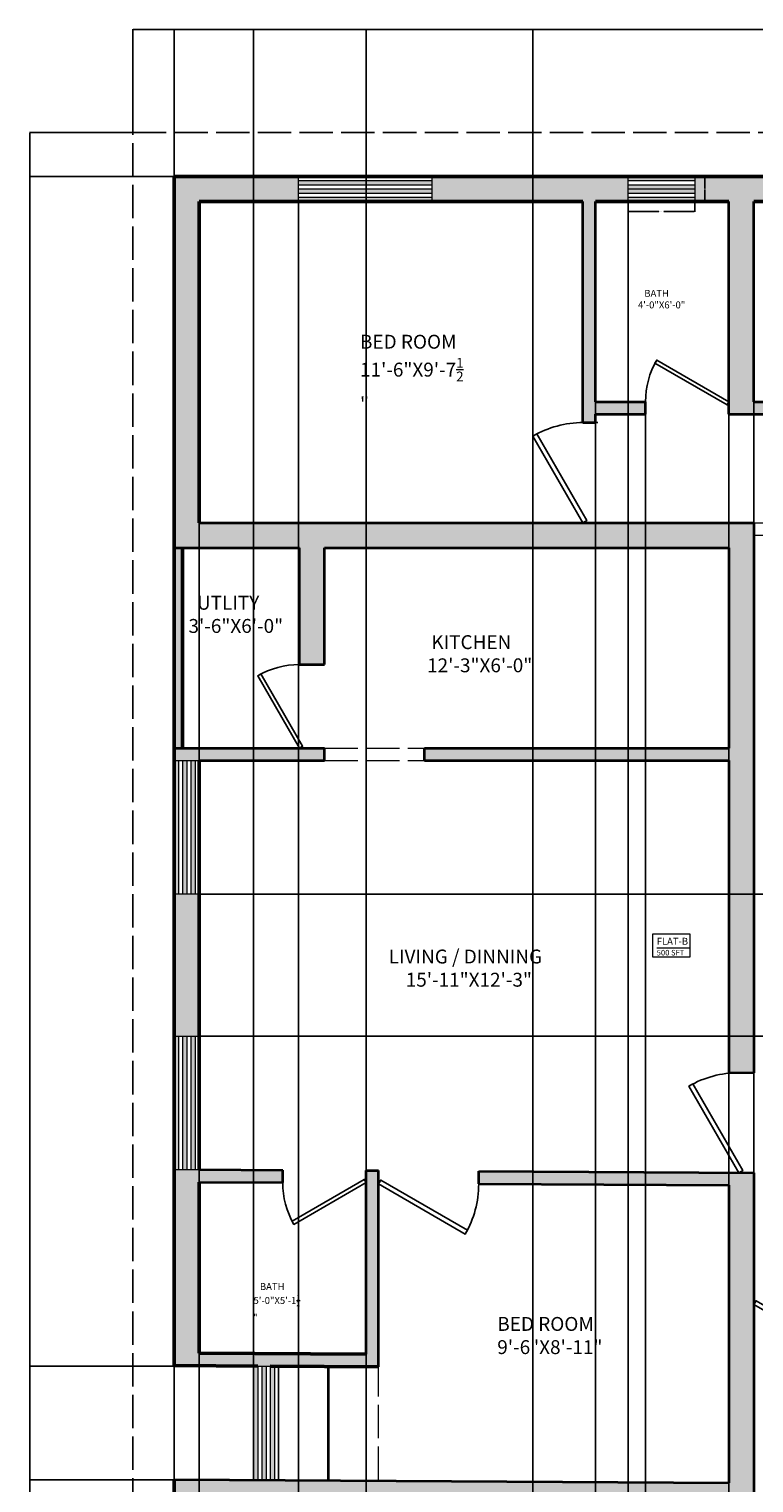
# Model space of a CAD drawing. Units: feet. Extents: x 2512 to 3087, y 1456 to 2266.
# Tile 3 of 5: x 2512 to 2773, y 1744 to 2266. Entities that reach past the tile are written whole.
import ezdxf

# ---------------------------------------------------------------- set-up
doc = ezdxf.new("R2010")
doc.units = ezdxf.units.FT
doc.linetypes.add('ACAD_ISO02W100', pattern=[15, 12, -3])
for name, color, linetype, lineweight in [('A-ANNO-DIMS', 2, 'Continuous', 18), ('A-AREA-IDEN', 7, 'Continuous', 18), ('A-DOOR', 240, 'Continuous', 25), ('A-GLAZ', 4, 'Continuous', 18), ('A-GLAZ-PATT', 252, 'Continuous', 13), ('A-WALL-OVHD', 8, 'ACAD_ISO02W100', 18), ('A-WALL-PATT', 252, 'Continuous', 13), ('ANNOTATION', 80, 'Continuous', 18), ('C-PROP', 8, 'ACAD_ISO02W100', 25), ('INNER WALL', 7, 'Continuous', 35), ('OPEN DOOR', 50, 'ACAD_ISO02W100', 18), ('OUTER WALL', 7, 'Continuous', 50)]:
    doc.layers.add(name, color=color, linetype=linetype, lineweight=lineweight)
doc.styles.get("Standard").update_dxf_attribs({"font": 'arial.ttf'})
doc.dimstyles.get("Standard").update_dxf_attribs({"dimtxt": 0.18, "dimasz": 0.18, "dimexe": 0.18, "dimexo": 0.0625, "dimgap": 0.09, "dimtad": 0, "dimtih": 1, "dimtoh": 1, "dimdec": 4, "dimzin": 0, "dimdsep": 46, "dimtxsty": 'Standard', "dimcen": 0.09, "dimadec": 0, "dimazin": 0, "dimtfac": 1, "dimtdec": 4, "dimtofl": 0, "dimtmove": 0, "dimatfit": 3, "dimfxl": 1, "dimtolj": 1, "dimtzin": 0, "dimarcsym": 0})

# ---------------------------------------------------------------- blocks, each defined once
blk = doc.blocks.new('*U8')
for p, q in [((0, 0), (0, 6)), ((40, 0), (40, 6))]:
    blk.add_line(p, q)
blk.add_lwpolyline([(0, 0), (34.64, -20), (35.52, -18.48), (0.87, 1.52)], close=True)
blk.add_arc((0, 0), 40, 330, 0)
blk = doc.blocks.new('*U3')
for p, q in [((0, 0), (0, 5)), ((40, 0), (40, 5))]:
    blk.add_line(p, q)
blk.add_lwpolyline([(0, 0), (34.64, -20), (35.52, -18.48), (0.87, 1.52)], close=True)
blk.add_arc((0, 0), 40, 330, 0)
blk = doc.blocks.new('*U4')
for p, q in [((-40, 0), (-40, 6)), ((0, 0), (0, 6))]:
    blk.add_line(p, q)
blk.add_lwpolyline([(0, 0), (-34.64, -20), (-35.52, -18.48), (-0.87, 1.52)], close=True)
blk.add_arc((0, 0), 40, 180, 210)
blk = doc.blocks.new('*U5')
for p, q in [((0, 0), (0, -6)), ((-40, 0), (-40, -6))]:
    blk.add_line(p, q)
blk.add_lwpolyline([(0, 0), (-34.64, 20), (-35.52, 18.48), (-0.88, -1.52)], close=True)
blk.add_arc((0, 0), 40, 150, 180)
blk = doc.blocks.new('*U6')
for p, q in [((-40, 0), (-40, 6)), ((0, 0), (0, 6))]:
    blk.add_line(p, q)
blk.add_lwpolyline([(0, 0), (-34.64, -20), (-35.52, -18.48), (-0.88, 1.52)], close=True)
blk.add_arc((0, 0), 40, 180, 210)
blk = doc.blocks.new('WIN-48IN')
h = blk.add_hatch(color=256)
h.dxf.hatch_style = 1
h.paths.add_polyline_path([(0, 7.5), (0, 6), (48, 6), (48, 7.5)])
h.paths.add_polyline_path([(48, 3), (48, 4.5), (0, 4.5), (0, 3)])
h.paths.add_polyline_path([(48, 0), (48, 1.5), (0, 1.5), (0, 0)])
for p, q in [((0, 9), (48, 9)), ((0, 0), (0, 9)), ((0, 7.5), (48, 7.5)), ((0, 6), (48, 6)), ((48, 9), (48, 0)), ((0, 4.5), (48, 4.5)), ((0, 4.5), (48, 4.5)), ((0, 3), (48, 3)), ((0, 1.5), (48, 1.5)), ((48, 0), (0, 0))]:
    blk.add_line(p, q)
blk = doc.blocks.new('VENT-24IN')
h = blk.add_hatch(color=256)
h.dxf.hatch_style = 1
h.paths.add_polyline_path([(24, 7.5), (24, 9), (0, 9), (0, 7.5)])
h.paths.add_polyline_path([(0, 1.5), (0, 0), (24, 0), (24, 1.5)])
h.paths.add_polyline_path([(0, 4.5), (0, 3), (24, 3), (24, 4.5)])
h.paths.add_polyline_path([(24, 4.5), (24, 6), (0, 6), (0, 4.5)])
for p, q in [((0, 9), (24, 9)), ((0, 0), (0, 9)), ((0, 7.5), (24, 7.5)), ((0, 6), (24, 6)), ((24, 9), (24, 0)), ((0, 4.5), (24, 4.5)), ((0, 3), (24, 3)), ((0, 1.5), (24, 1.5)), ((24, 0), (0, 0))]:
    blk.add_line(p, q)
blk = doc.blocks.new('FLAT-ID-FRAME')
blk.add_line((1.44, 3.36), (13.18, 3.36))
blk.add_lwpolyline([(0, 8.39), (13.37, 8.39), (13.37, 0), (0, 0)], close=True)
blk = doc.blocks.new('*D15')
at = {"layer": 'A-ANNO-DIMS', "color": 0, "lineweight": -2, "transparency": 16777216}
for p, q in [((2727.45, 2204.17), (2727.45, 2200.45)), ((2727.63, 2200.63), (2738.54, 2200.63)), ((2751.27, 2200.63), (2740.35, 2200.63)), ((2751.45, 2204.17), (2751.45, 2200.45))]:
    blk.add_line(p, q, dxfattribs=at)
at = {"layer": 'A-ANNO-DIMS', "color": 0, "transparency": 16777216}
for points in [[(2727.63, 2200.66), (2727.63, 2200.6), (2727.45, 2200.63)], [(2751.27, 2200.66), (2751.27, 2200.6), (2751.45, 2200.63)]]:
    blk.add_solid(points, dxfattribs=at)
at = {"layer": 'Defpoints', "color": 0, "transparency": 16777216}
for p in [(2727.45, 2204.23), (2751.45, 2204.23), (2751.45, 2200.63)]:
    blk.add_point(p, dxfattribs=at)
at = {"layer": 'A-ANNO-DIMS', "color": 0, "transparency": 16777216, "insert": (2739.45, 2200.63), "char_height": 0.18, "attachment_point": 5}
blk.add_mtext('\\A1;VENT 24 TYP.', dxfattribs=at)
blk = doc.blocks.new('*D16')
at = {"layer": 'A-ANNO-DIMS', "color": 0, "lineweight": -2, "transparency": 16777216}
for p, q in [((2751.51, 2213.23), (2755.23, 2213.23)), ((2755.05, 2213.05), (2755.05, 2208.91)), ((2755.05, 2204.41), (2755.05, 2208.55)), ((2751.51, 2204.23), (2755.23, 2204.23))]:
    blk.add_line(p, q, dxfattribs=at)
at = {"layer": 'A-ANNO-DIMS', "color": 0, "transparency": 16777216}
for points in [[(2755.02, 2213.05), (2755.08, 2213.05), (2755.05, 2213.23)], [(2755.02, 2204.41), (2755.08, 2204.41), (2755.05, 2204.23)]]:
    blk.add_solid(points, dxfattribs=at)
at = {"layer": 'Defpoints', "color": 0, "transparency": 16777216}
for p in [(2751.45, 2213.23), (2755.05, 2213.23), (2751.45, 2204.23)]:
    blk.add_point(p, dxfattribs=at)
at = {"layer": 'A-ANNO-DIMS', "color": 0, "transparency": 16777216, "insert": (2755.05, 2208.73), "char_height": 0.18, "attachment_point": 5}
blk.add_mtext('\\A1;9 TYP.', dxfattribs=at)
blk = doc.blocks.new('*D17')
at = {"layer": 'A-ANNO-DIMS', "color": 0, "lineweight": -2, "transparency": 16777216}
for p, q in [((2549.29, 2229.08), (2549.29, 2266.2)), ((2549.47, 2266.02), (2799.17, 2266.02)), ((3049.67, 2266.02), (2799.96, 2266.02)), ((3049.85, 2229.08), (3049.85, 2266.2))]:
    blk.add_line(p, q, dxfattribs=at)
at = {"layer": 'A-ANNO-DIMS', "color": 0, "transparency": 16777216}
for points in [[(2549.47, 2266.05), (2549.47, 2265.99), (2549.29, 2266.02)], [(3049.67, 2266.05), (3049.67, 2265.99), (3049.85, 2266.02)]]:
    blk.add_solid(points, dxfattribs=at)
at = {"layer": 'Defpoints', "color": 0, "transparency": 16777216}
for p in [(3049.85, 2266.02), (2549.29, 2229.02), (3049.85, 2229.02)]:
    blk.add_point(p, dxfattribs=at)
at = {"layer": 'A-ANNO-DIMS', "color": 0, "transparency": 16777216, "insert": (2799.57, 2266.02), "char_height": 0.18, "attachment_point": 5}
blk.add_mtext('\\A1;500.6', dxfattribs=at)
blk = doc.blocks.new('*D18')
at = {"layer": 'A-ANNO-DIMS', "color": 0, "lineweight": -2, "transparency": 16777216}
for p, q in [((2549.23, 2229.02), (2512.11, 2229.02)), ((2512.29, 2228.84), (2512.29, 1861.31)), ((2512.29, 1493.41), (2512.29, 1860.94)), ((2549.23, 1493.23), (2512.11, 1493.23))]:
    blk.add_line(p, q, dxfattribs=at)
at = {"layer": 'A-ANNO-DIMS', "color": 0, "transparency": 16777216}
for points in [[(2512.26, 2228.84), (2512.32, 2228.84), (2512.29, 2229.02)], [(2512.26, 1493.41), (2512.32, 1493.41), (2512.29, 1493.23)]]:
    blk.add_solid(points, dxfattribs=at)
at = {"layer": 'Defpoints', "color": 0, "transparency": 16777216}
for p in [(2512.29, 2229.02), (2549.29, 2229.02), (2549.29, 1493.23)]:
    blk.add_point(p, dxfattribs=at)
at = {"layer": 'A-ANNO-DIMS', "color": 0, "transparency": 16777216, "insert": (2512.29, 1861.13), "char_height": 0.18, "attachment_point": 5}
blk.add_mtext('\\A1;735.8', dxfattribs=at)
blk = doc.blocks.new('*D19')
at = {"layer": 'A-ANNO-DIMS', "color": 0, "lineweight": -2, "transparency": 16777216}
for p, q in [((2564.22, 2213.29), (2564.22, 2266.2)), ((2564.4, 2266.02), (2803.93, 2266.02)), ((3044.04, 2266.02), (2804.51, 2266.02)), ((3044.22, 2088.29), (3044.22, 2266.2))]:
    blk.add_line(p, q, dxfattribs=at)
at = {"layer": 'A-ANNO-DIMS', "color": 0, "transparency": 16777216}
for points in [[(2564.4, 2266.05), (2564.4, 2265.99), (2564.22, 2266.02)], [(3044.04, 2266.05), (3044.04, 2265.99), (3044.22, 2266.02)]]:
    blk.add_solid(points, dxfattribs=at)
at = {"layer": 'Defpoints', "color": 0, "transparency": 16777216}
for p in [(3044.22, 2266.02), (2564.22, 2213.23), (3044.22, 2088.23)]:
    blk.add_point(p, dxfattribs=at)
at = {"layer": 'A-ANNO-DIMS', "color": 0, "transparency": 16777216, "insert": (2804.22, 2266.02), "char_height": 0.18, "attachment_point": 5}
blk.add_mtext('\\A1;480', dxfattribs=at)
blk = doc.blocks.new('*D20')
at = {"layer": 'A-ANNO-DIMS', "color": 0, "lineweight": -2, "transparency": 16777216}
for p, q in [((2564.16, 2213.23), (2512.11, 2213.23)), ((2512.29, 2213.05), (2512.29, 1853.41)), ((2512.29, 1493.41), (2512.29, 1853.05)), ((2693.16, 1493.23), (2512.11, 1493.23))]:
    blk.add_line(p, q, dxfattribs=at)
at = {"layer": 'A-ANNO-DIMS', "color": 0, "transparency": 16777216}
for points in [[(2512.26, 2213.05), (2512.32, 2213.05), (2512.29, 2213.23)], [(2512.26, 1493.41), (2512.32, 1493.41), (2512.29, 1493.23)]]:
    blk.add_solid(points, dxfattribs=at)
at = {"layer": 'Defpoints', "color": 0, "transparency": 16777216}
for p in [(2512.29, 2213.23), (2564.22, 2213.23), (2693.22, 1493.23)]:
    blk.add_point(p, dxfattribs=at)
at = {"layer": 'A-ANNO-DIMS', "color": 0, "transparency": 16777216, "insert": (2512.29, 1853.23), "char_height": 0.18, "attachment_point": 5}
blk.add_mtext('\\A1;720', dxfattribs=at)
blk = doc.blocks.new('*D21')
at = {"layer": 'A-ANNO-DIMS', "color": 0, "lineweight": -2, "transparency": 16777216}
for p, q in [((2573.22, 2204.17), (2573.22, 1456.05)), ((2608.89, 2204.17), (2608.89, 1456.05)), ((2573.4, 1456.23), (2590.66, 1456.23)), ((2608.71, 1456.23), (2591.45, 1456.23))]:
    blk.add_line(p, q, dxfattribs=at)
at = {"layer": 'A-ANNO-DIMS', "color": 0, "transparency": 16777216}
for points in [[(2573.4, 1456.26), (2573.4, 1456.2), (2573.22, 1456.23)], [(2608.71, 1456.26), (2608.71, 1456.2), (2608.89, 1456.23)]]:
    blk.add_solid(points, dxfattribs=at)
at = {"layer": 'Defpoints', "color": 0, "transparency": 16777216}
for p in [(2573.22, 2204.23), (2608.89, 2204.23), (2608.89, 1456.23)]:
    blk.add_point(p, dxfattribs=at)
at = {"layer": 'A-ANNO-DIMS', "color": 0, "transparency": 16777216, "insert": (2591.05, 1456.23), "char_height": 0.18, "attachment_point": 5}
blk.add_mtext('\\A1;35.67', dxfattribs=at)
blk = doc.blocks.new('*D22')
at = {"layer": 'A-ANNO-DIMS', "color": 0, "lineweight": -2, "transparency": 16777216}
for p, q in [((2715.72, 2204.17), (2715.72, 1456.05)), ((2727.45, 2204.17), (2727.45, 1456.05)), ((2715.9, 1456.23), (2721.13, 1456.23)), ((2727.27, 1456.23), (2722.04, 1456.23))]:
    blk.add_line(p, q, dxfattribs=at)
at = {"layer": 'A-ANNO-DIMS', "color": 0, "transparency": 16777216}
for points in [[(2715.9, 1456.26), (2715.9, 1456.2), (2715.72, 1456.23)], [(2727.27, 1456.26), (2727.27, 1456.2), (2727.45, 1456.23)]]:
    blk.add_solid(points, dxfattribs=at)
at = {"layer": 'Defpoints', "color": 0, "transparency": 16777216}
for p in [(2715.72, 2204.23), (2727.45, 2204.23), (2727.45, 1456.23)]:
    blk.add_point(p, dxfattribs=at)
at = {"layer": 'A-ANNO-DIMS', "color": 0, "transparency": 16777216, "insert": (2721.58, 1456.23), "char_height": 0.18, "attachment_point": 5}
blk.add_mtext('\\A1;11.729', dxfattribs=at)
blk = doc.blocks.new('*D29')
at = {"layer": 'A-ANNO-DIMS', "color": 0, "lineweight": -2, "transparency": 16777216}
for p, q in [((2633.22, 1517.86), (2633.22, 2266.2)), ((2633.4, 2266.02), (2663, 2266.02)), ((2693.04, 2266.02), (2663.44, 2266.02)), ((2693.22, 1517.86), (2693.22, 2266.2))]:
    blk.add_line(p, q, dxfattribs=at)
at = {"layer": 'A-ANNO-DIMS', "color": 0, "transparency": 16777216}
for points in [[(2633.4, 2266.05), (2633.4, 2265.99), (2633.22, 2266.02)], [(2693.04, 2266.05), (2693.04, 2265.99), (2693.22, 2266.02)]]:
    blk.add_solid(points, dxfattribs=at)
at = {"layer": 'Defpoints', "color": 0, "transparency": 16777216}
for p in [(2693.22, 2266.02), (2633.22, 1517.8), (2693.22, 1517.8)]:
    blk.add_point(p, dxfattribs=at)
at = {"layer": 'A-ANNO-DIMS', "color": 0, "transparency": 16777216, "insert": (2663.22, 2266.02), "char_height": 0.18, "attachment_point": 5}
blk.add_mtext('\\A1;60', dxfattribs=at)
blk = doc.blocks.new('*D46')
at = {"layer": 'A-ANNO-DIMS', "color": 0, "lineweight": -2, "transparency": 16777216}
for p, q in [((2573.28, 1955.22), (3087.03, 1955.22)), ((3086.85, 1955.04), (3086.85, 1929.84)), ((3086.85, 1904.28), (3086.85, 1929.47)), ((2573.28, 1904.1), (3087.03, 1904.1))]:
    blk.add_line(p, q, dxfattribs=at)
at = {"layer": 'A-ANNO-DIMS', "color": 0, "transparency": 16777216}
for points in [[(3086.82, 1955.04), (3086.88, 1955.04), (3086.85, 1955.22)], [(3086.82, 1904.28), (3086.88, 1904.28), (3086.85, 1904.1)]]:
    blk.add_solid(points, dxfattribs=at)
at = {"layer": 'Defpoints', "color": 0, "transparency": 16777216}
for p in [(2573.22, 1955.22), (2573.22, 1904.1), (3086.85, 1904.1)]:
    blk.add_point(p, dxfattribs=at)
at = {"layer": 'A-ANNO-DIMS', "color": 0, "transparency": 16777216, "insert": (3086.85, 1929.66), "char_height": 0.18, "attachment_point": 5}
blk.add_mtext('\\A1;51.12', dxfattribs=at)
blk = doc.blocks.new('*D47')
at = {"layer": 'A-ANNO-DIMS', "color": 0, "lineweight": -2, "transparency": 16777216}
for p, q in [((2592.66, 1785.56), (2512.11, 1785.56)), ((2512.29, 1785.38), (2512.29, 1765.3)), ((2512.29, 1744.86), (2512.29, 1764.94)), ((2592.66, 1744.68), (2512.11, 1744.68))]:
    blk.add_line(p, q, dxfattribs=at)
at = {"layer": 'A-ANNO-DIMS', "color": 0, "transparency": 16777216}
for points in [[(2512.26, 1785.38), (2512.32, 1785.38), (2512.29, 1785.56)], [(2512.26, 1744.86), (2512.32, 1744.86), (2512.29, 1744.68)]]:
    blk.add_solid(points, dxfattribs=at)
at = {"layer": 'Defpoints', "color": 0, "transparency": 16777216}
for p in [(2512.29, 1785.56), (2592.72, 1785.56), (2592.72, 1744.68)]:
    blk.add_point(p, dxfattribs=at)
at = {"layer": 'A-ANNO-DIMS', "color": 0, "transparency": 16777216, "insert": (2512.29, 1765.12), "char_height": 0.18, "attachment_point": 5}
blk.add_mtext('\\A1;40.89', dxfattribs=at)
blk = doc.blocks.new('*D48')
at = {"layer": 'A-ANNO-DIMS', "color": 0, "lineweight": -2, "transparency": 16777216}
for p, q in [((2564.22, 1744.79), (2564.22, 2266.2)), ((2564.4, 2266.02), (2578.14, 2266.02)), ((2592.54, 2266.02), (2578.79, 2266.02)), ((2592.72, 1744.74), (2592.72, 2266.2))]:
    blk.add_line(p, q, dxfattribs=at)
at = {"layer": 'A-ANNO-DIMS', "color": 0, "transparency": 16777216}
for points in [[(2564.4, 2266.05), (2564.4, 2265.99), (2564.22, 2266.02)], [(2592.54, 2266.05), (2592.54, 2265.99), (2592.72, 2266.02)]]:
    blk.add_solid(points, dxfattribs=at)
at = {"layer": 'Defpoints', "color": 0, "transparency": 16777216}
for p in [(2564.22, 2266.02), (2564.22, 1744.73), (2592.72, 1744.68)]:
    blk.add_point(p, dxfattribs=at)
at = {"layer": 'A-ANNO-DIMS', "color": 0, "transparency": 16777216, "insert": (2578.47, 2266.02), "char_height": 0.18, "attachment_point": 5}
blk.add_mtext('\\A1;28.5', dxfattribs=at)
blk = doc.blocks.new('*D53')
at = {"layer": 'A-ANNO-DIMS', "color": 0, "lineweight": -2, "transparency": 16777216}
for p, q in [((2733.72, 2127.67), (2733.72, 1456.05)), ((2763.72, 2127.67), (2763.72, 1456.05)), ((2733.9, 1456.23), (2748.5, 1456.23)), ((2763.54, 1456.23), (2748.94, 1456.23))]:
    blk.add_line(p, q, dxfattribs=at)
at = {"layer": 'A-ANNO-DIMS', "color": 0, "transparency": 16777216}
for points in [[(2733.9, 1456.26), (2733.9, 1456.2), (2733.72, 1456.23)], [(2763.54, 1456.26), (2763.54, 1456.2), (2763.72, 1456.23)]]:
    blk.add_solid(points, dxfattribs=at)
at = {"layer": 'Defpoints', "color": 0, "transparency": 16777216}
for p in [(2733.72, 2127.73), (2763.72, 2127.73), (2763.72, 1456.23)]:
    blk.add_point(p, dxfattribs=at)
at = {"layer": 'A-ANNO-DIMS', "color": 0, "transparency": 16777216, "insert": (2748.72, 1456.23), "char_height": 0.18, "attachment_point": 5}
blk.add_mtext('\\A1;30', dxfattribs=at)
blk = doc.blocks.new('*D54')
at = {"layer": 'A-ANNO-DIMS', "color": 0, "lineweight": -2, "transparency": 16777216}
for p, q in [((2763.72, 2127.67), (2763.72, 1456.05)), ((2772.72, 2132.17), (2772.72, 1456.05)), ((2763.9, 1456.23), (2768.07, 1456.23)), ((2772.54, 1456.23), (2768.37, 1456.23))]:
    blk.add_line(p, q, dxfattribs=at)
at = {"layer": 'A-ANNO-DIMS', "color": 0, "transparency": 16777216}
for points in [[(2763.9, 1456.26), (2763.9, 1456.2), (2763.72, 1456.23)], [(2772.54, 1456.26), (2772.54, 1456.2), (2772.72, 1456.23)]]:
    blk.add_solid(points, dxfattribs=at)
at = {"layer": 'Defpoints', "color": 0, "transparency": 16777216}
for p in [(2763.72, 2127.73), (2772.72, 2132.23), (2772.72, 1456.23)]:
    blk.add_point(p, dxfattribs=at)
at = {"layer": 'A-ANNO-DIMS', "color": 0, "transparency": 16777216, "insert": (2768.22, 1456.23), "char_height": 0.18, "attachment_point": 5}
blk.add_mtext('\\A1;9', dxfattribs=at)

msp = doc.modelspace()

# ---------------------------------------------------------------- hatches: boundary and pattern name
at = {"layer": 'A-GLAZ-PATT'}
h = msp.add_hatch(color=256, dxfattribs=at)
h.dxf.hatch_style = 1
h.paths.add_polyline_path([(2600.2185, 1785.5197), (2598.7185, 1785.5284), (2598.7185, 1744.6752), (2600.2185, 1744.6752)])
h.paths.add_polyline_path([(2597.2185, 1785.5371), (2595.7185, 1785.5458), (2595.7185, 1744.6752), (2597.2185, 1744.6752)])
h.paths.add_polyline_path([(2594.2185, 1785.5544), (2592.7185, 1785.5631), (2592.7185, 1744.6752), (2594.2185, 1744.6752)])
at = {"layer": 'A-WALL-PATT'}
h = msp.add_hatch(color=256, dxfattribs=at)
h.dxf.hatch_style = 1
h.paths.add_polyline_path([(3035.2185, 1915.2872), (3026.2185, 1915.2872), (3026.2185, 1912.7316), (2936.2185, 1912.7316), (2936.2185, 2001.7316), (2931.7185, 2001.7316), (2931.7185, 1912.7316), (2808.7185, 1912.7316), (2808.7185, 1903.7316), (3026.2185, 1903.7316), (3026.2185, 1816.7316), (2808.7185, 1816.7316), (2808.7185, 1807.7316), (2823.7185, 1807.7316), (2823.7185, 1638.2316), (2828.2185, 1638.2316), (2828.2185, 1674.2316), (2828.2185, 1678.7316), (2828.2185, 1807.7316), (3026.2185, 1807.7316), (3026.2185, 1735.7316), (3002.2185, 1735.7316), (3002.2546, 1726.7316), (3011.2546, 1726.7316), (3035.2185, 1726.7316)])
h.paths.add_polyline_path([(3035.2185, 2001.7316), (2990.2185, 2001.7316), (2972.2185, 2001.7316), (2972.2185, 1996.7316), (3026.2185, 1996.7316), (3026.2185, 1963.2872), (3035.2185, 1963.2872)], flags=17)
h.paths.add_polyline_path([(3041.2185, 2010.7316), (2990.2185, 2010.7316), (2990.2185, 2001.7316), (3035.2185, 2001.7316), (3041.2185, 2001.7316)])
h.paths.add_polyline_path([(3044.2185, 2085.7316), (3044.2185, 2088.2316), (3041.2185, 2088.2316), (3041.2185, 2006.2316), (3044.2185, 2006.2316)])
h.paths.add_polyline_path([(3041.2185, 2090.2316), (2975.2185, 2090.2316), (2975.2185, 2090.2254), (2966.2185, 2090.2254), (2825.2185, 2090.2316), (2825.2185, 2091.7316), (2820.7185, 2091.7316), (2820.7185, 2085.7316), (2820.7185, 2084.2316), (2825.2185, 2084.2316), (2825.2185, 2085.7316), (2990.2185, 2085.7316), (2990.2185, 2046.7316), (2999.2185, 2046.7316), (2999.2185, 2085.7316), (3041.2185, 2085.7316)])
h.paths.add_polyline_path([(3035.2185, 2213.2316), (2918.3922, 2213.2316), (2918.3922, 2204.2316), (3026.2185, 2204.2316), (3026.2185, 2144.2316), (2966.2185, 2144.2316), (2966.2185, 2135.213), (2975.2185, 2135.213), (2975.2185, 2135.2316), (3035.2185, 2135.2316)])
h.paths.add_polyline_path([(2870.3922, 2213.2316), (2809.1404, 2213.2316), (2809.1404, 2204.2316), (2820.7185, 2204.2316), (2820.7185, 2162.2316), (2825.2185, 2162.2316), (2825.2185, 2204.2316), (2870.3922, 2204.2316)])
h.paths.add_polyline_path([(2785.1404, 2213.2316), (2751.447, 2213.2316), (2751.447, 2204.2316), (2763.7185, 2204.2316), (2763.7185, 2127.7316), (2825.2185, 2127.7316), (2825.2185, 2132.2316), (2820.7185, 2132.2316), (2772.7185, 2132.2316), (2772.7185, 2204.2316), (2785.1404, 2204.2316)])
h.paths.add_polyline_path([(2727.447, 2213.2316), (2656.8898, 2213.2316), (2656.8898, 2204.2316), (2711.2185, 2204.2316), (2711.2185, 2124.7316), (2715.7185, 2124.7316), (2715.7185, 2127.7316), (2733.7185, 2127.7316), (2733.7185, 2132.2316), (2715.7185, 2132.2316), (2715.7185, 2204.2316), (2727.447, 2204.2316)], flags=17)
h.paths.add_polyline_path([(2608.8898, 2213.2316), (2564.2185, 2213.2316), (2564.2185, 2079.7316), (2609.2185, 2079.7316), (2609.2185, 2037.7316), (2618.2185, 2037.7316), (2618.2185, 2079.7316), (2763.7185, 2079.7316), (2763.7185, 2007.7316), (2654.2185, 2007.7316), (2654.2185, 2003.2316), (2763.7185, 2003.2316), (2763.7185, 1891.0755), (2772.7185, 1891.0234), (2772.7185, 1903.7316), (2772.7185, 2088.7316), (2573.2185, 2088.7316), (2573.2185, 2204.2316), (2608.8898, 2204.2316)])
h.paths.add_polyline_path([(2567.2185, 2079.7316), (2564.2185, 2079.7316), (2564.2185, 2007.7316), (2567.2185, 2007.7316)], flags=17)
h.paths.add_polyline_path([(2618.2185, 2007.7316), (2564.2185, 2007.7316), (2564.2185, 2003.2171), (2573.2185, 2003.2171), (2573.2185, 2003.2316), (2618.2185, 2003.2316)], flags=17)
h.paths.add_polyline_path([(2573.2185, 1955.2171), (2564.2185, 1955.2171), (2564.2185, 1904.096), (2573.2185, 1904.096)], flags=17)
h.paths.add_polyline_path([(2573.2185, 1851.677), (2603.2185, 1851.5035), (2603.2195, 1856.0035), (2573.2185, 1856.1771), (2573.2185, 1856.096), (2564.2185, 1856.096), (2564.2185, 1785.728), (2594.2185, 1785.5544), (2600.2185, 1785.5197), (2637.7185, 1785.3028), (2637.7185, 1855.8039), (2633.2185, 1855.83), (2633.2185, 1789.8289), (2573.2185, 1790.176)])
h.paths.add_polyline_path([(2772.7185, 1855.0228), (2767.3185, 1855.0228), (2767.3004, 1855.0542), (2673.7185, 1855.5956), (2673.7185, 1851.0956), (2763.7185, 1850.575), (2763.7185, 1743.5732), (2564.2185, 1744.7273), (2564.2185, 1719.3702), (2573.2185, 1719.3702), (2573.2185, 1735.6751), (2633.2185, 1735.328), (2633.2185, 1717.3272), (2637.7185, 1717.3272), (2637.7185, 1735.302), (2772.7185, 1734.521)])
h.paths.add_polyline_path([(2697.7185, 1734.9549), (2693.2185, 1734.9809), (2693.2185, 1602.8011), (2697.7185, 1602.8011)])
h.paths.add_polyline_path([(2823.7185, 1561.2231), (2733.7185, 1561.7437), (2733.7185, 1552.7436), (2823.7185, 1552.2229)])
h.paths.add_polyline_path([(2697.7185, 1566.8011), (2693.2185, 1566.8011), (2693.2185, 1562.8011), (2682.4194, 1562.8011), (2682.4194, 1553.8011), (2693.2185, 1553.8011), (2693.2185, 1495.2316), (2697.7185, 1495.2316)])
h.paths.add_polyline_path([(2828.2185, 1495.2316), (2693.2185, 1495.2316), (2693.2185, 1493.2316), (2828.2185, 1493.2316)])
h.paths.add_polyline_path([(2828.2185, 1602.2316), (2823.7185, 1602.2316), (2823.7185, 1495.2316), (2828.2185, 1495.2316)])
h.paths.add_polyline_path([(3035.2185, 1523.0765), (3026.2185, 1523.0765), (3026.2185, 1513.7316), (2828.2185, 1513.7316), (2828.2185, 1504.7316), (3035.2185, 1504.7316)])
h.paths.add_polyline_path([(3026.2185, 1602.2316), (2906.2185, 1602.2316), (2906.2185, 1644.2316), (2901.7185, 1644.2316), (2901.7185, 1597.7316), (3026.2185, 1597.7316)])
h.paths.add_polyline_path([(3035.2185, 1678.7316), (2864.2185, 1678.7316), (2864.2185, 1674.2316), (3026.2185, 1674.2316), (3026.2185, 1642.5123), (3035.2185, 1642.5123)], flags=17)
h.paths.add_polyline_path([(3035.2185, 1618.5123), (3026.2185, 1618.5123), (3026.2185, 1571.0765), (3035.2185, 1571.0765)])
h = msp.add_hatch(color=256, dxfattribs=at)
h.dxf.hatch_style = 1
h.paths.add_polyline_path([(2573.2185, 2204.2316), (2608.8898, 2204.2316), (2608.8898, 2213.2316), (2564.2185, 2213.2316), (2564.2185, 2079.7316), (2609.2185, 2079.7316), (2609.2185, 2037.7316), (2613.7185, 2037.7316), (2618.2185, 2037.7316), (2618.2185, 2079.7316), (2763.7185, 2079.7316), (2763.7185, 2007.7316), (2654.2185, 2007.7316), (2654.2185, 2003.2316), (2763.7185, 2003.2316), (2763.7185, 1891.0755), (2772.7185, 1891.0234), (2772.7185, 1903.7316), (2772.7185, 2088.7316), (2573.2185, 2088.7316)])
h.paths.add_polyline_path([(2727.447, 2213.2316), (2656.8898, 2213.2316), (2656.8898, 2204.2316), (2711.2185, 2204.2316), (2711.2185, 2124.7316), (2715.7185, 2124.7316), (2715.7185, 2127.7316), (2733.7185, 2127.7316), (2733.7185, 2132.2316), (2715.7185, 2132.2316), (2715.7185, 2204.2316), (2727.447, 2204.2316)], flags=17)
h.paths.add_polyline_path([(2785.1404, 2213.2316), (2751.447, 2213.2316), (2751.447, 2204.2316), (2763.7185, 2204.2316), (2763.7185, 2127.7316), (2825.2185, 2127.7316), (2825.2185, 2132.2316), (2820.7185, 2132.2316), (2772.7185, 2132.2316), (2772.7185, 2204.2316), (2785.1404, 2204.2316)])
h.paths.add_polyline_path([(2966.2185, 2204.2316), (2825.2185, 2204.2316), (2825.2185, 2162.2316), (2820.7185, 2162.2316, 0.12053744), (2806.8695, 2158.8438), (2822.234, 2132.2316), (2825.2185, 2132.2316), (2825.2185, 2127.7316), (2826.1185, 2127.7316, -0.12053744), (2842.7373, 2123.6662), (2842.7545, 2123.696), (2844.1185, 2122.9085), (2826.1185, 2091.7316), (2825.2185, 2091.7316), (2825.2185, 2090.2316), (2966.2185, 2090.2316), (2966.2185, 2135.213), (2966.2185, 2144.2316)], flags=17)
h.paths.add_polyline_path([(2870.3922, 2213.2316), (2809.1404, 2213.2316), (2809.1404, 2204.2316), (2820.7185, 2204.2316), (2820.7185, 2162.2316), (2825.2185, 2162.2316), (2825.2185, 2204.2316), (2870.3922, 2204.2316)])
h.paths.add_polyline_path([(3035.2185, 2213.2316), (2918.3922, 2213.2316), (2918.3922, 2204.2316), (3026.2185, 2204.2316), (3026.2185, 2144.2316), (2966.2185, 2144.2316), (2966.2185, 2135.213), (2975.2185, 2135.213), (2975.2185, 2135.2316), (3035.2185, 2135.2316)])
h.paths.add_polyline_path([(2999.2185, 2085.7316), (3041.2185, 2085.7316), (3041.2185, 2090.2316), (2975.2185, 2090.2316), (2975.2185, 2090.2254), (2966.2185, 2090.2254), (2825.2185, 2090.2316), (2825.2185, 2091.7316), (2820.7185, 2091.7316), (2820.7185, 2085.7316), (2820.7185, 2084.2316), (2825.2185, 2084.2316), (2825.2185, 2085.7316), (2990.2185, 2085.7316), (2990.2185, 2046.7316), (2995.6185, 2046.7316), (2999.2185, 2046.7316)])
h.paths.add_polyline_path([(3041.2185, 2010.7316), (2990.2185, 2010.7316), (2990.2185, 2001.7316), (3041.2185, 2001.7316)])
h.paths.add_polyline_path([(3035.2185, 2001.7316), (2990.2185, 2001.7316), (2972.2185, 2001.7316), (2972.2185, 1996.7316), (3026.2185, 1996.7316), (3026.2185, 1963.2872), (3035.2185, 1963.2872)])
h.paths.add_polyline_path([(3044.2185, 2085.7316), (3044.2185, 2088.2316), (3041.2185, 2088.2316), (3041.2185, 2085.7316), (3041.2185, 2006.2316), (3044.2185, 2006.2316)])
h.paths.add_polyline_path([(2966.2185, 2135.213), (2966.2185, 2144.2316), (2966.2185, 2204.2316), (2918.3922, 2204.2316), (2825.2185, 2204.2316), (2825.2185, 2162.2316), (2820.7185, 2162.2316, 0.12053744), (2806.8695, 2158.8438), (2822.234, 2132.2316), (2825.2185, 2132.2316), (2825.2185, 2127.7316), (2826.1185, 2127.7316, -0.12053744), (2842.7373, 2123.6662), (2842.7545, 2123.696), (2844.1185, 2122.9085), (2826.1185, 2091.7316), (2825.2185, 2091.7316), (2825.2185, 2090.2316), (2966.2185, 2090.2316)], flags=17)
h.paths.add_polyline_path([(2869.2463, 2140.1407), (2910.0273, 2140.1407), (2910.0273, 2158.8321), (2869.2463, 2158.8321)], flags=8)
h = msp.add_hatch(color=256, dxfattribs=at)
h.dxf.hatch_style = 1
h.paths.add_polyline_path([(2573.2185, 1683.1742), (2637.6925, 1682.8012), (2637.6947, 1687.3013), (2573.2185, 1687.6743), (2573.2185, 1695.3702), (2564.2185, 1695.3702), (2564.2185, 1517.8011), (2624.2185, 1517.8011), (2633.2185, 1517.8011), (2633.2185, 1553.8011), (2634.4194, 1553.8011), (2634.4194, 1562.8011), (2624.2185, 1562.8011), (2624.2185, 1526.8011), (2573.2185, 1526.8011)])
h.paths.add_polyline_path([(2573.2185, 1735.6751), (2633.2185, 1735.328), (2633.2185, 1717.3272), (2637.7096, 1717.3272), (2637.7185, 1735.302), (2772.7185, 1734.521), (2772.7185, 1855.0228), (2673.7185, 1855.5956), (2673.7185, 1851.0956), (2763.7185, 1850.575), (2763.7185, 1743.5732), (2564.2185, 1744.7273), (2564.2185, 1719.3702), (2573.2185, 1719.3702)])
h.paths.add_polyline_path([(2828.2185, 1807.7316), (3026.2185, 1807.7316), (3026.2185, 1735.7316), (3002.2185, 1735.7316), (3002.2546, 1726.7316), (3011.2546, 1726.7316), (3035.2185, 1726.7316), (3035.2185, 1915.2872), (3026.2185, 1915.2872), (3026.2185, 1912.7316), (2936.2185, 1912.7316), (2936.2185, 2001.7316), (2931.7185, 2001.7316), (2931.7185, 1912.7316), (2808.7185, 1912.7316), (2808.7185, 1903.7316), (3026.2185, 1903.7316), (3026.2185, 1816.7316), (2808.7185, 1816.7316), (2808.7185, 1807.7316), (2823.7185, 1807.7316), (2823.7185, 1638.2316), (2828.2185, 1638.2316), (2828.2185, 1674.2316), (2828.2185, 1678.7316)])
h.paths.add_polyline_path([(3035.2185, 1678.7316), (2864.2185, 1678.7316), (2864.2185, 1674.2316), (3026.2185, 1674.2316), (3026.2185, 1642.5123), (3035.2185, 1642.5123)], flags=17)
h.paths.add_polyline_path([(3035.2185, 1618.5123), (3026.2185, 1618.5123), (3026.2185, 1571.0765), (3035.2185, 1571.0765)])
h.paths.add_polyline_path([(3026.2185, 1602.2316), (2906.2185, 1602.2316), (2906.2185, 1644.2316), (2901.7185, 1644.2316), (2901.7185, 1597.7316), (3026.2185, 1597.7316)])
h.paths.add_polyline_path([(3035.2185, 1523.0765), (3026.2185, 1523.0765), (3026.2185, 1513.7316), (2828.2185, 1513.7316), (2828.2185, 1504.7316), (3035.2185, 1504.7316)])
h.paths.add_polyline_path([(2828.2185, 1495.2316), (2693.2185, 1495.2316), (2693.2185, 1493.2316), (2828.2185, 1493.2316)])
h.paths.add_polyline_path([(2828.2185, 1602.2316), (2823.7185, 1602.2316), (2823.7185, 1495.2316), (2828.2185, 1495.2316)])
h.paths.add_polyline_path([(2823.7185, 1561.2231), (2733.7185, 1561.7437), (2733.7185, 1552.7436), (2823.7185, 1552.2229)])
h.paths.add_polyline_path([(2697.7185, 1566.8011), (2693.2185, 1566.8011), (2693.2185, 1562.8011), (2682.4194, 1562.8011), (2682.4194, 1553.8011), (2693.2185, 1553.8011), (2693.2185, 1495.2316), (2697.7185, 1495.2316)])
h.paths.add_polyline_path([(2697.7185, 1734.9549), (2693.2185, 1734.9809), (2693.2185, 1602.8011), (2697.7185, 1602.8011)])
h.paths.add_polyline_path([(2573.2185, 1851.677), (2603.2185, 1851.5035), (2603.2195, 1856.0035), (2573.2185, 1856.1771), (2573.2185, 1856.096), (2564.2185, 1856.096), (2564.2185, 1785.728), (2594.2185, 1785.5544), (2600.2185, 1785.5197), (2637.7185, 1785.3028), (2637.7185, 1855.8039), (2633.2185, 1855.83), (2633.2185, 1789.8289), (2573.2185, 1790.176)])
h.paths.add_polyline_path([(2573.2185, 1955.2171), (2564.2185, 1955.2171), (2564.2185, 1904.096), (2573.2185, 1904.096)])
h.paths.add_polyline_path([(2618.2185, 2007.7316), (2564.2185, 2007.7316), (2564.2185, 2003.2171), (2573.2185, 2003.2171), (2573.2185, 2003.2316), (2618.2185, 2003.2316)])
h.paths.add_polyline_path([(2567.2185, 2079.7316), (2564.2185, 2079.7316), (2564.2185, 2007.7316), (2567.2185, 2007.7316)])

# ---------------------------------------------------------------- linework, layer by layer
at = {"layer": 'A-GLAZ'}
for p, q in [((2592.7185, 1744.6752), (2592.7185, 1785.5631)), ((2592.7185, 1785.5631), (2600.2185, 1785.5197)), ((2592.7185, 1744.6752), (2592.7185, 1785.3028)), ((2594.2185, 1785.5544), (2594.2185, 1744.6752)), ((2595.7185, 1785.5458), (2595.7185, 1744.6752)), ((2595.7185, 1785.5458), (2597.2185, 1785.5371)), ((2597.2185, 1785.5371), (2597.2185, 1744.6752)), ((2597.2185, 1785.5371), (2597.2185, 1744.6752)), ((2598.7185, 1785.5284), (2598.7185, 1744.6752)), ((2600.2185, 1785.5197), (2600.2185, 1744.6752)), ((2601.7185, 1785.5111), (2601.7185, 1744.6752)), ((2601.7185, 1744.6752), (2601.7185, 1785.3028)), ((2601.7185, 1744.6752), (2592.7185, 1744.6752))]:
    msp.add_line(p, q, dxfattribs=at)
at = {"layer": 'A-WALL-OVHD'}
for p, q in [((2564.2185, 1785.728), (2564.2185, 1744.7273)), ((2637.7185, 1744.6752), (2637.7185, 1785.3028))]:
    msp.add_line(p, q, dxfattribs=at)
at = {"layer": 'C-PROP'}
for p, q in [((2549.289, 1493.2316), (2549.289, 2229.0217)), ((2549.289, 2229.0217), (3049.8469, 2229.0217))]:
    msp.add_line(p, q, dxfattribs=at)
at = {"layer": 'INNER WALL'}
for p, q in [((2711.2185, 2124.7316), (2711.2185, 2204.2316)), ((2715.7185, 2132.2316), (2715.7185, 2204.2316)), ((2763.7185, 2127.7316), (2763.7185, 2204.2316)), ((2772.7185, 2132.2316), (2772.7185, 2204.2316)), ((2715.7185, 2132.2316), (2733.7185, 2132.2316)), ((2715.7185, 2124.7316), (2715.7185, 2127.7316)), ((2715.7185, 2127.7316), (2733.7185, 2127.7316)), ((2715.7185, 2127.7316), (2733.7185, 2127.7316)), ((2733.7185, 2127.7316), (2733.7185, 2132.2316)), ((2763.7185, 2127.7316), (2825.2185, 2127.7316)), ((2772.7185, 2132.2316), (2825.2185, 2132.2316)), ((2711.2185, 2124.7316), (2715.7185, 2124.7316)), ((2573.2185, 2088.7316), (2772.7185, 2088.7316)), ((2772.7185, 2088.7316), (2772.7185, 1903.7316)), ((2564.2185, 2079.7316), (2609.2185, 2079.7316)), ((2609.2185, 2037.7316), (2609.2185, 2079.7316)), ((2618.2185, 2079.7316), (2763.7185, 2079.7316)), ((2618.2185, 2037.7316), (2618.2185, 2079.7316)), ((2763.7185, 2079.7316), (2763.7185, 2007.7316)), ((2609.2185, 2037.7316), (2618.2185, 2037.7316)), ((2564.2185, 2007.7316), (2618.2185, 2007.7316)), ((2618.2185, 2003.2316), (2618.2185, 2007.7316)), ((2654.2185, 2007.7316), (2763.7185, 2007.7316)), ((2654.2185, 2003.2316), (2654.2185, 2007.7316)), ((2573.2185, 2003.2316), (2618.2185, 2003.2316)), ((2654.2185, 2003.2316), (2763.7185, 2003.2316)), ((2763.7185, 2003.2316), (2763.7185, 1891.0755)), ((2772.7185, 1903.7316), (2772.7185, 1891.0234)), ((2763.7185, 1891.0755), (2772.9268, 1891.0222)), ((2573.2185, 1856.1771), (2603.2195, 1856.0035)), ((2603.2185, 1851.5035), (2603.2195, 1856.0035)), ((2633.2185, 1789.8289), (2633.2185, 1855.83)), ((2633.2185, 1855.83), (2637.7185, 1855.8039)), ((2637.7185, 1785.3028), (2637.7185, 1855.8039)), ((2673.7185, 1851.0956), (2673.7185, 1855.5956)), ((2673.7185, 1855.5956), (2772.7185, 1855.0228)), ((2573.2185, 1851.677), (2603.2185, 1851.5035)), ((2673.7185, 1851.0956), (2763.7185, 1850.575)), ((2763.7185, 1850.575), (2763.7185, 1743.5732)), ((2772.7185, 1855.0228), (2772.7185, 1734.521)), ((2603.2185, 1789.8289), (2603.2185, 1790.0025)), ((2619.7185, 1744.6752), (2619.7185, 1785.3028)), ((2564.2185, 1744.7273), (2763.7185, 1743.5732))]:
    msp.add_line(p, q, dxfattribs=at)
at = {"layer": 'OPEN DOOR'}
for p, q in [((2772.7185, 2088.7316), (2820.7185, 2088.7316)), ((2772.7185, 2084.2316), (2825.2185, 2084.2316)), ((2618.2185, 2007.7316), (2654.2185, 2007.7316)), ((2618.2185, 2003.2316), (2654.2185, 2003.2316))]:
    msp.add_line(p, q, dxfattribs=at)
at = {"layer": 'OUTER WALL'}
for p, q in [((2564.2185, 2213.2316), (3035.2185, 2213.2316)), ((2564.2185, 1785.728), (2564.2185, 2213.2316)), ((2573.2185, 2204.2316), (2711.2185, 2204.2316)), ((2573.2185, 2088.7316), (2573.2185, 2204.2316)), ((2715.7185, 2204.2316), (2763.7185, 2204.2316)), ((2772.7185, 2204.2316), (2820.7185, 2204.2316)), ((2567.2185, 2007.7316), (2567.2185, 2079.7316)), ((2573.2185, 1856.1771), (2573.2185, 2003.2316)), ((2573.2185, 1790.176), (2573.2185, 1851.677)), ((2573.2185, 1790.176), (2633.2185, 1789.8289)), ((2564.2185, 1785.728), (2594.2185, 1785.5544)), ((2598.7185, 1785.5284), (2637.7185, 1785.3028)), ((2564.2185, 1517.8011), (2564.2185, 1744.7273))]:
    msp.add_line(p, q, dxfattribs=at)

# ---------------------------------------------------------------- block references
at = {"layer": 'A-AREA-IDEN'}
msp.add_blockref('FLAT-ID-FRAME', (2736.3118, 1932.5554), dxfattribs=at)
at = {"layer": 'A-DOOR'}
for name, p, xscale, yscale, zscale in [('*U5', (2763.7185, 2132.2316), 0.7500000000000038, 0.7500000000000038, 0.7500000000000038), ('*U6', (2633.2185, 1851.5035), 0.7500000000000038, 0.7500000000000038, 0.7500000000000038), ('*U3', (2637.7185, 1851.0212), 0.899999999999959, 0.899999999999959, 0.899999999999959), ('*U8', (2772.7185, 1807.692), 0.899999999999959, 0.899999999999959, 0.899999999999959)]:
    msp.add_blockref(name, p, dxfattribs=dict(at, xscale=xscale, yscale=yscale, zscale=zscale))
at = {"layer": 'A-DOOR', "rotation": 270}
for name, p, xscale, yscale, zscale in [('*U4', (2711.2185, 2088.7316), 0.899999999999959, 0.899999999999959, 0.899999999999959), ('*U6', (2609.2185, 2007.7316), 0.7500000000000038, 0.7500000000000038, 0.7500000000000038), ('*U6', (2767.3185, 1855.0228), 0.899999999999959, 0.899999999999959, 0.899999999999959)]:
    msp.add_blockref(name, p, dxfattribs=dict(at, xscale=xscale, yscale=yscale, zscale=zscale))
at = {"layer": 'A-GLAZ'}
for name, p in [('WIN-48IN', (2608.89, 2204.232)), ('VENT-24IN', (2727.447, 2204.232))]:
    msp.add_blockref(name, p, dxfattribs=at)
for p, rotation in [((2564.2189, 2003.2169), 269.9999999999981), ((2564.2189, 1904.0958), 269.9999999999968)]:
    msp.add_blockref('WIN-48IN', p, dxfattribs=dict(at, rotation=rotation))

# ---------------------------------------------------------------- texts
at = {"layer": 'A-AREA-IDEN', "attachment_point": 1}
for s, width, insert, char_height in [('FLAT-B', 12.525641, (2737.7535, 1939.5155), 2.5), ('500 SFT', 11.390914, (2737.7535, 1935.173), 2)]:
    msp.add_mtext_dynamic_manual_height_columns(s, width=width, gutter_width=12.5, heights=[0], dxfattribs=dict(at, insert=insert, char_height=char_height))
at = {"layer": 'ANNOTATION', "attachment_point": 1}
for s, width, insert, char_height in [('   BATH\\P4\'-0"X6\'-0"', 16.842597, (2730.9978, 2172.4527), 2.5), ('\\A1;BED ROOM\\P11\'-6"X9\'-7{\\H0.7x;\\S1/2;}"', 38.558323, (2631.0164, 2156.3031), 5), ('\\A1;  UTLITY\\P3\'-6"X6\'-0"', 38.558323, (2569.3235, 2062.4656), 5), ('\\A1; KITCHEN\\P12\'-3"X6\'-0"', 38.558323, (2655.155, 2048.3075), 5), ('\\A1;LIVING / DINNING\\P    15\'-11"X12\'-3"', 59.172495, (2641.3555, 1935.2817), 5), ('\\A1;   BATH\\P5\'-0"X5\'-1{\\H0.7x;\\S1/2;}"', 16.842597, (2592.7185, 1815.4088), 2.5), ('\\A1;BED ROOM\\P9\'-6"X8\'-11"', 38.558323, (2680.4, 1803.202), 5)]:
    msp.add_mtext_dynamic_manual_height_columns(s, width=width, gutter_width=12.5, heights=[0], dxfattribs=dict(at, insert=insert, char_height=char_height))

# ---------------------------------------------------------------- dimensions: what is measured, and where the dimension line sits
at = {"layer": 'A-ANNO-DIMS'}
for base, p1, p2, override, picture, middle in [((3049.8469, 2266.0217), (2549.289, 2229.0217), (3049.8469, 2229.0217), {"dimdec": 1, "dimlfac": 1, "dimrnd": 0, "dimzin": 0, "dimdsep": 46, "dimlunit": 2}, '*D17', (2799.5679, 2266.0217)), ((3044.2185, 2266.0217), (2564.2185, 2213.2316), (3044.2185, 2088.2316), {"dimdec": 0, "dimlfac": 1, "dimrnd": 0, "dimzin": 0, "dimdsep": 46, "dimlunit": 2}, '*D19', (2804.2185, 2266.0217)), ((2564.2185, 2266.0217), (2592.7185, 1744.6752), (2564.2185, 1744.7273), {"dimdec": 1, "dimlfac": 1, "dimrnd": 0, "dimzin": 0, "dimdsep": 46, "dimlunit": 2}, '*D48', (2578.4685, 2266.0217)), ((2693.2185, 2266.0217), (2633.2185, 1517.8011), (2693.2185, 1517.8011), {"dimdec": 0, "dimlfac": 1, "dimrnd": 0, "dimzin": 0, "dimdsep": 46, "dimlunit": 2}, '*D29', (2663.2185, 2266.0217)), ((2608.8898, 1456.2316), (2573.2185, 2204.2316), (2608.8898, 2204.2316), {"dimdec": 2, "dimlfac": 1, "dimrnd": 0, "dimzin": 0, "dimdsep": 46, "dimlunit": 2}, '*D21', (2591.0541, 1456.2316)), ((2727.44702, 1456.23162), (2715.71848, 2204.23162), (2727.44702, 2204.23162), {"dimdec": 3, "dimlfac": 1, "dimrnd": 0, "dimzin": 0, "dimdsep": 46, "dimlunit": 2}, '*D22', (2721.58275, 1456.23162)), ((2763.7185, 1456.2316), (2733.7185, 2127.7316), (2763.7185, 2127.7316), {"dimdec": 0, "dimlfac": 1, "dimrnd": 0, "dimzin": 0, "dimdsep": 46, "dimlunit": 2}, '*D53', (2748.7185, 1456.2316)), ((2772.7185, 1456.2316), (2763.7185, 2127.7316), (2772.7185, 2132.2316), {"dimdec": 0, "dimlfac": 1, "dimrnd": 0, "dimzin": 0, "dimdsep": 46, "dimlunit": 2}, '*D54', (2768.2185, 1456.2316))]:
    dim = msp.add_linear_dim(base=base, p1=p1, p2=p2, dimstyle='Standard', override=override, dxfattribs=at)
    dim.commit()
    dim.dimension.update_dxf_attribs({"geometry": picture, "text_midpoint": middle})
for base, p1, p2, override, picture, middle in [((2512.289, 2229.0217), (2549.289, 1493.2316), (2549.289, 2229.0217), {"dimdec": 1, "dimlfac": 1, "dimrnd": 0, "dimzin": 0, "dimdsep": 46, "dimlunit": 2}, '*D18', (2512.289, 1861.1267)), ((2512.289, 2213.2316), (2693.2185, 1493.2316), (2564.2185, 2213.2316), {"dimdec": 0, "dimlfac": 1, "dimrnd": 0, "dimzin": 0, "dimdsep": 46, "dimlunit": 2}, '*D20', (2512.289, 1853.2316)), ((3086.8469, 1904.096), (2573.2185, 1955.2171), (2573.2185, 1904.096), {"dimdec": 2, "dimlfac": 1, "dimrnd": 0, "dimzin": 0, "dimdsep": 46, "dimlunit": 2}, '*D46', (3086.8469, 1929.6566)), ((2512.289, 1785.5631), (2592.7185, 1744.6752), (2592.7185, 1785.5631), {"dimdec": 2, "dimlfac": 1, "dimrnd": 0, "dimzin": 0, "dimdsep": 46, "dimlunit": 2}, '*D47', (2512.289, 1765.1192))]:
    dim = msp.add_linear_dim(base=base, p1=p1, p2=p2, angle=90, dimstyle='Standard', override=override, dxfattribs=at)
    dim.commit()
    dim.dimension.update_dxf_attribs({"geometry": picture, "text_midpoint": middle})
dim = msp.add_linear_dim(base=(2755.047, 2213.2316), p1=(2751.447, 2204.2316), p2=(2751.447, 2213.2316), angle=90, text='<> TYP.', dimstyle='Standard', override={"dimdec": 0, "dimlfac": 1, "dimrnd": 0, "dimzin": 0, "dimdsep": 46, "dimlunit": 2}, dxfattribs=at)
dim.commit()
dim.dimension.update_dxf_attribs({"geometry": '*D16', "text_midpoint": (2755.047, 2208.7316)})
dim = msp.add_linear_dim(base=(2751.447, 2200.6316), p1=(2727.447, 2204.2316), p2=(2751.447, 2204.2316), text='VENT <> TYP.', dimstyle='Standard', override={"dimdec": 0, "dimlfac": 1, "dimrnd": 0, "dimzin": 0, "dimdsep": 46, "dimlunit": 2}, dxfattribs=at)
dim.commit()
dim.dimension.update_dxf_attribs({"geometry": '*D15', "text_midpoint": (2739.447, 2200.6316)})

doc.saveas('drawing.dxf')
